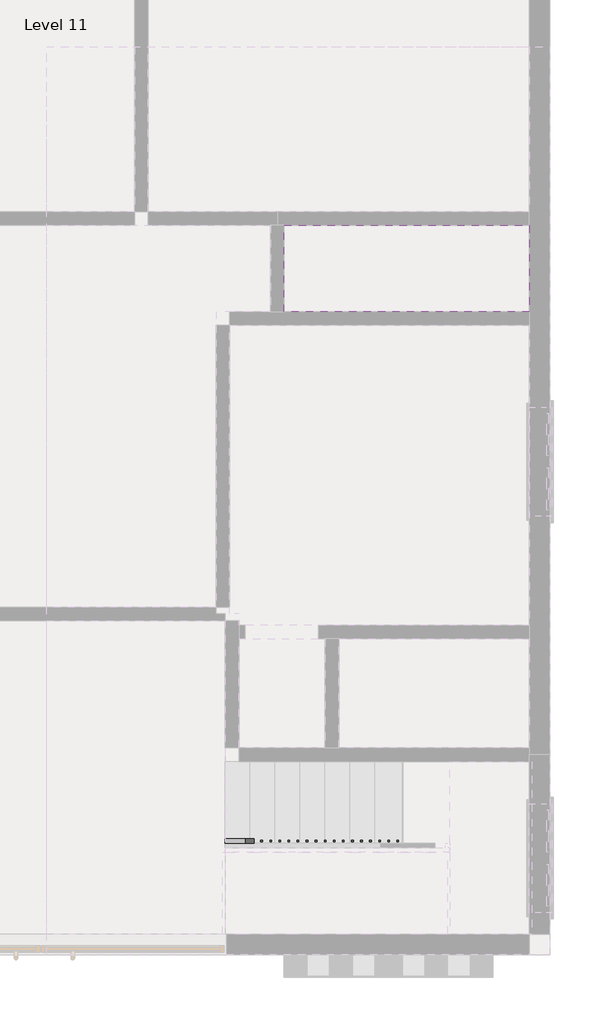
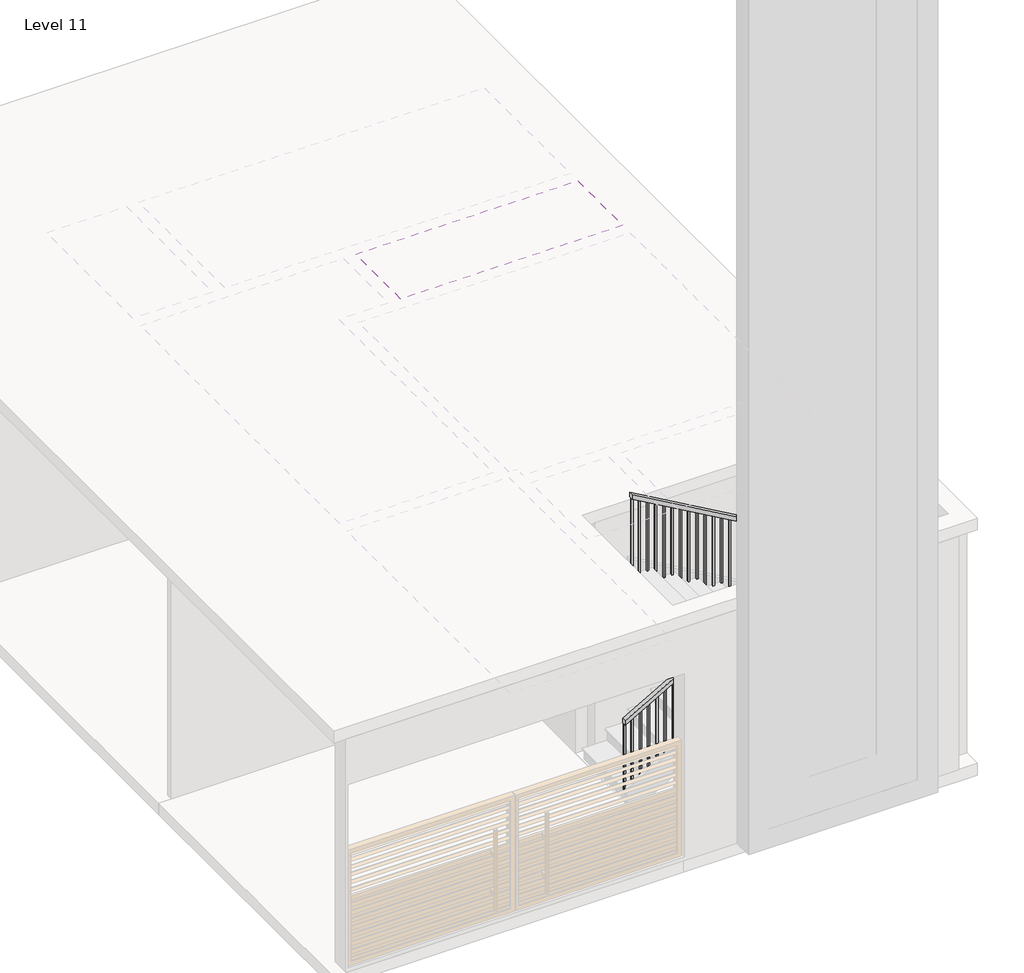
# One storey, part 2 of 3: 2 railings, 1 covering.
"""IFC4 building model written with IfcOpenShell, lengths in millimetres."""

from ifc_helpers import new_model, si_unit, frame, origin, place, context, project, spatial, polyline, outline, extrude, faceted_brep, element, save

model = new_model("IFC4")

# Units and contexts
model_context = context("Model", 3, world=origin())
ifc_project = project(units=[si_unit("LENGTHUNIT", "METRE", prefix="MILLI")], contexts=[model_context])

# Site, building, storey
site = spatial("IfcSite", under=ifc_project)
building = spatial("IfcBuilding", under=site)
storey = spatial("IfcBuildingStorey", under=building, Name="Level 11", Elevation=0.0)

# Covering
placement = place(None, origin())
element("IfcCovering", 1, ObjectType="2' x 4' ACT System", at=placement, inside=storey, context=model_context, shape_type="SweptSolid", body=[
    extrude(outline(polyline([(-930.7154463, 2171.4455275), (1812.4845537, 2171.4455275), (1812.4845537, 1206.2455275), (-930.7154463, 1206.2455275), (-930.7154463, 2171.4455275)])), frame((0.0, 0.0, 2743.2), z_axis=(0.0, 0.0, 1.0), x_axis=(1.0, 0.0, 0.0)), (0.0, 0.0, 1.0), 57.15),
])

# Railings
element("IfcRailing", 2, ObjectType="Handrail - Rectangular", at=placement, inside=storey, context=model_context, shape_type="SolidModel", body=[
    faceted_brep([(-1591.1154463, -4686.5544725, 1074.42), (-1591.1154463, -4686.5544725, 1015.8782835), (-1591.1154463, -4737.3544725, 1015.8782835), (-1591.1154463, -4737.3544725, 1074.42), (847.2845537, -4686.5544725, 2470.9581818), (898.0845537, -4686.5544725, 2441.5110107), (898.0845537, -4737.3544725, 2441.5110107), (847.2845537, -4737.3544725, 2470.9581818), (847.2845537, -4686.5544725, 2514.6), (898.0845537, -4686.5544725, 2463.8), (898.0845537, -4737.3544725, 2463.8), (847.2845537, -4737.3544725, 2514.6), (974.2845537, -4686.5544725, 2514.6), (974.2845537, -4686.5544725, 2463.8), (923.4845537, -4737.3544725, 2463.8), (923.4845537, -4737.3544725, 2514.6), (974.2845537, -4813.5544725, 2514.6), (974.2845537, -4813.5544725, 2463.8), (923.4845537, -4813.5544725, 2463.8), (923.4845537, -4813.5544725, 2514.6), (974.2845537, -4838.9544725, 2514.6), (923.4845537, -4838.9544725, 2514.6), (923.4845537, -4889.7544725, 2463.8), (974.2845537, -4889.7544725, 2463.8)], [[[0, 1, 2, 3]], [[1, 0, 4, 5]], [[2, 1, 5, 6]], [[3, 2, 6, 7]], [[0, 3, 7, 4]], [[5, 4, 8, 9]], [[6, 5, 9, 10]], [[7, 6, 10, 11]], [[4, 7, 11, 8]], [[9, 8, 12, 13]], [[10, 9, 13, 14]], [[11, 10, 14, 15]], [[8, 11, 15, 12]], [[13, 12, 16, 17]], [[14, 13, 17, 18]], [[15, 14, 18, 19]], [[12, 15, 19, 16]], [[20, 21, 22, 23]], [[17, 16, 20, 23]], [[18, 17, 23, 22]], [[19, 18, 22, 21]], [[16, 19, 21, 20]]]),
    faceted_brep([(974.2845537, -4838.9544725, 2514.6), (974.2845537, -4889.7544725, 2463.8), (923.4845537, -4889.7544725, 2463.8), (923.4845537, -4838.9544725, 2514.6), (974.2845537, -4838.9544725, 2645.5254545), (923.4845537, -4838.9544725, 2616.0782835), (923.4845537, -4889.7544725, 2616.0782835), (974.2845537, -4889.7544725, 2645.5254545)], [[[0, 1, 2, 3]], [[4, 5, 6, 7]], [[1, 0, 4, 7]], [[2, 1, 7, 6]], [[3, 2, 6, 5]], [[0, 3, 5, 4]]]),
    faceted_brep([(974.2845537, -4889.7544725, 2645.5254545), (923.4845537, -4889.7544725, 2616.0782835), (923.4845537, -4838.9544725, 2616.0782835), (974.2845537, -4838.9544725, 2645.5254545), (-1591.1154463, -4889.7544725, 4114.8), (-1591.1154463, -4838.9544725, 4114.8), (-1591.1154463, -4838.9544725, 4056.2582835), (-1591.1154463, -4889.7544725, 4056.2582835)], [[[0, 1, 2, 3]], [[4, 5, 6, 7]], [[1, 0, 4, 7]], [[2, 1, 7, 6]], [[3, 2, 6, 5]], [[0, 3, 5, 4]]]),
    extrude(outline(polyline([(3992.6139653, -1479.9904463), (4003.5244198, -1499.0404463), (3040.38, -1499.0404463), (3040.38, -1479.9904463), (3992.6139653, -1479.9904463)])), frame((0.0, -4873.8794725, 0.0), z_axis=(0.0, 1.0, 0.0), x_axis=(0.0, 0.0, 1.0)), (0.0, 0.0, 1.0), 19.05),
    extrude(outline(polyline([(3934.4248744, -1378.3904463), (3945.3353289, -1397.4404463), (3040.38, -1397.4404463), (3040.38, -1378.3904463), (3934.4248744, -1378.3904463)])), frame((0.0, -4873.8794725, 0.0), z_axis=(0.0, 1.0, 0.0), x_axis=(0.0, 0.0, 1.0)), (0.0, 0.0, 1.0), 19.05),
    extrude(outline(polyline([(3876.2357835, -1276.7904463), (3887.146238, -1295.8404463), (2880.36, -1295.8404463), (2880.36, -1276.7904463), (3876.2357835, -1276.7904463)])), frame((0.0, -4873.8794725, 0.0), z_axis=(0.0, 1.0, 0.0), x_axis=(0.0, 0.0, 1.0)), (0.0, 0.0, 1.0), 19.05),
    extrude(outline(polyline([(3818.0466926, -1175.1904463), (3828.9571471, -1194.2404463), (2880.36, -1194.2404463), (2880.36, -1175.1904463), (3818.0466926, -1175.1904463)])), frame((0.0, -4873.8794725, 0.0), z_axis=(0.0, 1.0, 0.0), x_axis=(0.0, 0.0, 1.0)), (0.0, 0.0, 1.0), 19.05),
    extrude(outline(polyline([(3759.8576016, -1073.5904463), (3770.7680562, -1092.6404463), (2880.36, -1092.6404463), (2880.36, -1073.5904463), (3759.8576016, -1073.5904463)])), frame((0.0, -4873.8794725, 0.0), z_axis=(0.0, 1.0, 0.0), x_axis=(0.0, 0.0, 1.0)), (0.0, 0.0, 1.0), 19.05),
    extrude(outline(polyline([(3701.6685107, -971.9904463), (3712.5789653, -991.0404463), (2720.34, -991.0404463), (2720.34, -971.9904463), (3701.6685107, -971.9904463)])), frame((0.0, -4873.8794725, 0.0), z_axis=(0.0, 1.0, 0.0), x_axis=(0.0, 0.0, 1.0)), (0.0, 0.0, 1.0), 19.05),
    extrude(outline(polyline([(3643.4794198, -870.3904463), (3654.3898744, -889.4404463), (2720.34, -889.4404463), (2720.34, -870.3904463), (3643.4794198, -870.3904463)])), frame((0.0, -4873.8794725, 0.0), z_axis=(0.0, 1.0, 0.0), x_axis=(0.0, 0.0, 1.0)), (0.0, 0.0, 1.0), 19.05),
    extrude(outline(polyline([(3585.2903289, -768.7904463), (3596.2007835, -787.8404463), (2720.34, -787.8404463), (2720.34, -768.7904463), (3585.2903289, -768.7904463)])), frame((0.0, -4873.8794725, 0.0), z_axis=(0.0, 1.0, 0.0), x_axis=(0.0, 0.0, 1.0)), (0.0, 0.0, 1.0), 19.05),
    extrude(outline(polyline([(3527.101238, -667.1904463), (3538.0116926, -686.2404463), (2560.32, -686.2404463), (2560.32, -667.1904463), (3527.101238, -667.1904463)])), frame((0.0, -4873.8794725, 0.0), z_axis=(0.0, 1.0, 0.0), x_axis=(0.0, 0.0, 1.0)), (0.0, 0.0, 1.0), 19.05),
    extrude(outline(polyline([(3468.9121471, -565.5904463), (3479.8226016, -584.6404463), (2560.32, -584.6404463), (2560.32, -565.5904463), (3468.9121471, -565.5904463)])), frame((0.0, -4873.8794725, 0.0), z_axis=(0.0, 1.0, 0.0), x_axis=(0.0, 0.0, 1.0)), (0.0, 0.0, 1.0), 19.05),
    extrude(outline(polyline([(3410.7230562, -463.9904463), (3421.6335107, -483.0404463), (2560.32, -483.0404463), (2560.32, -463.9904463), (3410.7230562, -463.9904463)])), frame((0.0, -4873.8794725, 0.0), z_axis=(0.0, 1.0, 0.0), x_axis=(0.0, 0.0, 1.0)), (0.0, 0.0, 1.0), 19.05),
    extrude(outline(polyline([(3352.5339653, -362.3904463), (3363.4444198, -381.4404463), (2400.3, -381.4404463), (2400.3, -362.3904463), (3352.5339653, -362.3904463)])), frame((0.0, -4873.8794725, 0.0), z_axis=(0.0, 1.0, 0.0), x_axis=(0.0, 0.0, 1.0)), (0.0, 0.0, 1.0), 19.05),
    extrude(outline(polyline([(3294.3448744, -260.7904463), (3305.2553289, -279.8404463), (2400.3, -279.8404463), (2400.3, -260.7904463), (3294.3448744, -260.7904463)])), frame((0.0, -4873.8794725, 0.0), z_axis=(0.0, 1.0, 0.0), x_axis=(0.0, 0.0, 1.0)), (0.0, 0.0, 1.0), 19.05),
    extrude(outline(polyline([(3236.1557835, -159.1904463), (3247.066238, -178.2404463), (2240.28, -178.2404463), (2240.28, -159.1904463), (3236.1557835, -159.1904463)])), frame((0.0, -4873.8794725, 0.0), z_axis=(0.0, 1.0, 0.0), x_axis=(0.0, 0.0, 1.0)), (0.0, 0.0, 1.0), 19.05),
    extrude(outline(polyline([(3177.9666926, -57.5904463), (3188.8771471, -76.6404463), (2240.28, -76.6404463), (2240.28, -57.5904463), (3177.9666926, -57.5904463)])), frame((0.0, -4873.8794725, 0.0), z_axis=(0.0, 1.0, 0.0), x_axis=(0.0, 0.0, 1.0)), (0.0, 0.0, 1.0), 19.05),
    extrude(outline(polyline([(3119.7776016, 44.0095537), (3130.6880562, 24.9595537), (2240.28, 24.9595537), (2240.28, 44.0095537), (3119.7776016, 44.0095537)])), frame((0.0, -4873.8794725, 0.0), z_axis=(0.0, 1.0, 0.0), x_axis=(0.0, 0.0, 1.0)), (0.0, 0.0, 1.0), 19.05),
    extrude(outline(polyline([(3061.5885107, 145.6095537), (3072.4989653, 126.5595537), (2080.26, 126.5595537), (2080.26, 145.6095537), (3061.5885107, 145.6095537)])), frame((0.0, -4873.8794725, 0.0), z_axis=(0.0, 1.0, 0.0), x_axis=(0.0, 0.0, 1.0)), (0.0, 0.0, 1.0), 19.05),
    extrude(outline(polyline([(3003.3994198, 247.2095537), (3014.3098744, 228.1595537), (2080.26, 228.1595537), (2080.26, 247.2095537), (3003.3994198, 247.2095537)])), frame((0.0, -4873.8794725, 0.0), z_axis=(0.0, 1.0, 0.0), x_axis=(0.0, 0.0, 1.0)), (0.0, 0.0, 1.0), 19.05),
    extrude(outline(polyline([(2945.2103289, 348.8095537), (2956.1207835, 329.7595537), (2080.26, 329.7595537), (2080.26, 348.8095537), (2945.2103289, 348.8095537)])), frame((0.0, -4873.8794725, 0.0), z_axis=(0.0, 1.0, 0.0), x_axis=(0.0, 0.0, 1.0)), (0.0, 0.0, 1.0), 19.05),
    extrude(outline(polyline([(2887.021238, 450.4095537), (2897.9316926, 431.3595537), (1920.24, 431.3595537), (1920.24, 450.4095537), (2887.021238, 450.4095537)])), frame((0.0, -4873.8794725, 0.0), z_axis=(0.0, 1.0, 0.0), x_axis=(0.0, 0.0, 1.0)), (0.0, 0.0, 1.0), 19.05),
    extrude(outline(polyline([(2828.8321471, 552.0095537), (2839.7426016, 532.9595537), (1920.24, 532.9595537), (1920.24, 552.0095537), (2828.8321471, 552.0095537)])), frame((0.0, -4873.8794725, 0.0), z_axis=(0.0, 1.0, 0.0), x_axis=(0.0, 0.0, 1.0)), (0.0, 0.0, 1.0), 19.05),
    extrude(outline(polyline([(2770.6430562, 653.6095537), (2781.5535107, 634.5595537), (1920.24, 634.5595537), (1920.24, 653.6095537), (2770.6430562, 653.6095537)])), frame((0.0, -4873.8794725, 0.0), z_axis=(0.0, 1.0, 0.0), x_axis=(0.0, 0.0, 1.0)), (0.0, 0.0, 1.0), 19.05),
    extrude(outline(polyline([(2712.4539653, 755.2095537), (2723.3644198, 736.1595537), (1760.22, 736.1595537), (1760.22, 755.2095537), (2712.4539653, 755.2095537)])), frame((0.0, -4873.8794725, 0.0), z_axis=(0.0, 1.0, 0.0), x_axis=(0.0, 0.0, 1.0)), (0.0, 0.0, 1.0), 19.05),
    extrude(outline(polyline([(2654.2648744, 856.8095537), (2665.1753289, 837.7595537), (1760.22, 837.7595537), (1760.22, 856.8095537), (2654.2648744, 856.8095537)])), frame((0.0, -4873.8794725, 0.0), z_axis=(0.0, 1.0, 0.0), x_axis=(0.0, 0.0, 1.0)), (0.0, 0.0, 1.0), 19.05),
    extrude(outline(polyline([(939.3595537, -4804.0294725), (958.4095537, -4804.0294725), (958.4095537, -4823.0794725), (939.3595537, -4823.0794725), (939.3595537, -4804.0294725)])), frame((0.0, 0.0, 1600.2), z_axis=(0.0, 0.0, 1.0), x_axis=(1.0, 0.0, 0.0)), (0.0, 0.0, 1.0), 863.6),
    extrude(outline(polyline([(2417.8716926, 856.8095537), (2406.961238, 837.7595537), (1440.18, 837.7595537), (1440.18, 856.8095537), (2417.8716926, 856.8095537)])), frame((0.0, -4721.4794725, 0.0), z_axis=(0.0, 1.0, 0.0), x_axis=(0.0, 0.0, 1.0)), (0.0, 0.0, 1.0), 19.05),
    extrude(outline(polyline([(2359.6826016, 755.2095537), (2348.7721471, 736.1595537), (1440.18, 736.1595537), (1440.18, 755.2095537), (2359.6826016, 755.2095537)])), frame((0.0, -4721.4794725, 0.0), z_axis=(0.0, 1.0, 0.0), x_axis=(0.0, 0.0, 1.0)), (0.0, 0.0, 1.0), 19.05),
    extrude(outline(polyline([(2301.4935107, 653.6095537), (2290.5830562, 634.5595537), (1440.18, 634.5595537), (1440.18, 653.6095537), (2301.4935107, 653.6095537)])), frame((0.0, -4721.4794725, 0.0), z_axis=(0.0, 1.0, 0.0), x_axis=(0.0, 0.0, 1.0)), (0.0, 0.0, 1.0), 19.05),
    extrude(outline(polyline([(2243.3044198, 552.0095537), (2232.3939653, 532.9595537), (1280.16, 532.9595537), (1280.16, 552.0095537), (2243.3044198, 552.0095537)])), frame((0.0, -4721.4794725, 0.0), z_axis=(0.0, 1.0, 0.0), x_axis=(0.0, 0.0, 1.0)), (0.0, 0.0, 1.0), 19.05),
    extrude(outline(polyline([(2185.1153289, 450.4095537), (2174.2048744, 431.3595537), (1280.16, 431.3595537), (1280.16, 450.4095537), (2185.1153289, 450.4095537)])), frame((0.0, -4721.4794725, 0.0), z_axis=(0.0, 1.0, 0.0), x_axis=(0.0, 0.0, 1.0)), (0.0, 0.0, 1.0), 19.05),
    extrude(outline(polyline([(2126.926238, 348.8095537), (2116.0157835, 329.7595537), (1120.14, 329.7595537), (1120.14, 348.8095537), (2126.926238, 348.8095537)])), frame((0.0, -4721.4794725, 0.0), z_axis=(0.0, 1.0, 0.0), x_axis=(0.0, 0.0, 1.0)), (0.0, 0.0, 1.0), 19.05),
    extrude(outline(polyline([(2068.7371471, 247.2095537), (2057.8266926, 228.1595537), (1120.14, 228.1595537), (1120.14, 247.2095537), (2068.7371471, 247.2095537)])), frame((0.0, -4721.4794725, 0.0), z_axis=(0.0, 1.0, 0.0), x_axis=(0.0, 0.0, 1.0)), (0.0, 0.0, 1.0), 19.05),
    extrude(outline(polyline([(2010.5480562, 145.6095537), (1999.6376016, 126.5595537), (1120.14, 126.5595537), (1120.14, 145.6095537), (2010.5480562, 145.6095537)])), frame((0.0, -4721.4794725, 0.0), z_axis=(0.0, 1.0, 0.0), x_axis=(0.0, 0.0, 1.0)), (0.0, 0.0, 1.0), 19.05),
    extrude(outline(polyline([(1952.3589653, 44.0095537), (1941.4485107, 24.9595537), (960.12, 24.9595537), (960.12, 44.0095537), (1952.3589653, 44.0095537)])), frame((0.0, -4721.4794725, 0.0), z_axis=(0.0, 1.0, 0.0), x_axis=(0.0, 0.0, 1.0)), (0.0, 0.0, 1.0), 19.05),
    extrude(outline(polyline([(1894.1698744, -57.5904463), (1883.2594198, -76.6404463), (960.12, -76.6404463), (960.12, -57.5904463), (1894.1698744, -57.5904463)])), frame((0.0, -4721.4794725, 0.0), z_axis=(0.0, 1.0, 0.0), x_axis=(0.0, 0.0, 1.0)), (0.0, 0.0, 1.0), 19.05),
    extrude(outline(polyline([(1835.9807835, -159.1904463), (1825.0703289, -178.2404463), (960.12, -178.2404463), (960.12, -159.1904463), (1835.9807835, -159.1904463)])), frame((0.0, -4721.4794725, 0.0), z_axis=(0.0, 1.0, 0.0), x_axis=(0.0, 0.0, 1.0)), (0.0, 0.0, 1.0), 19.05),
    extrude(outline(polyline([(1777.7916926, -260.7904463), (1766.881238, -279.8404463), (800.1, -279.8404463), (800.1, -260.7904463), (1777.7916926, -260.7904463)])), frame((0.0, -4721.4794725, 0.0), z_axis=(0.0, 1.0, 0.0), x_axis=(0.0, 0.0, 1.0)), (0.0, 0.0, 1.0), 19.05),
    extrude(outline(polyline([(1719.6026016, -362.3904463), (1708.6921471, -381.4404463), (800.1, -381.4404463), (800.1, -362.3904463), (1719.6026016, -362.3904463)])), frame((0.0, -4721.4794725, 0.0), z_axis=(0.0, 1.0, 0.0), x_axis=(0.0, 0.0, 1.0)), (0.0, 0.0, 1.0), 19.05),
    extrude(outline(polyline([(1661.4135107, -463.9904463), (1650.5030562, -483.0404463), (800.1, -483.0404463), (800.1, -463.9904463), (1661.4135107, -463.9904463)])), frame((0.0, -4721.4794725, 0.0), z_axis=(0.0, 1.0, 0.0), x_axis=(0.0, 0.0, 1.0)), (0.0, 0.0, 1.0), 19.05),
    extrude(outline(polyline([(1603.2244198, -565.5904463), (1592.3139653, -584.6404463), (640.08, -584.6404463), (640.08, -565.5904463), (1603.2244198, -565.5904463)])), frame((0.0, -4721.4794725, 0.0), z_axis=(0.0, 1.0, 0.0), x_axis=(0.0, 0.0, 1.0)), (0.0, 0.0, 1.0), 19.05),
    extrude(outline(polyline([(1545.0353289, -667.1904463), (1534.1248744, -686.2404463), (640.08, -686.2404463), (640.08, -667.1904463), (1545.0353289, -667.1904463)])), frame((0.0, -4721.4794725, 0.0), z_axis=(0.0, 1.0, 0.0), x_axis=(0.0, 0.0, 1.0)), (0.0, 0.0, 1.0), 19.05),
    extrude(outline(polyline([(1486.846238, -768.7904463), (1475.9357835, -787.8404463), (480.06, -787.8404463), (480.06, -768.7904463), (1486.846238, -768.7904463)])), frame((0.0, -4721.4794725, 0.0), z_axis=(0.0, 1.0, 0.0), x_axis=(0.0, 0.0, 1.0)), (0.0, 0.0, 1.0), 19.05),
    extrude(outline(polyline([(1428.6571471, -870.3904463), (1417.7466926, -889.4404463), (480.06, -889.4404463), (480.06, -870.3904463), (1428.6571471, -870.3904463)])), frame((0.0, -4721.4794725, 0.0), z_axis=(0.0, 1.0, 0.0), x_axis=(0.0, 0.0, 1.0)), (0.0, 0.0, 1.0), 19.05),
    extrude(outline(polyline([(1370.4680562, -971.9904463), (1359.5576016, -991.0404463), (480.06, -991.0404463), (480.06, -971.9904463), (1370.4680562, -971.9904463)])), frame((0.0, -4721.4794725, 0.0), z_axis=(0.0, 1.0, 0.0), x_axis=(0.0, 0.0, 1.0)), (0.0, 0.0, 1.0), 19.05),
    extrude(outline(polyline([(1312.2789653, -1073.5904463), (1301.3685107, -1092.6404463), (320.04, -1092.6404463), (320.04, -1073.5904463), (1312.2789653, -1073.5904463)])), frame((0.0, -4721.4794725, 0.0), z_axis=(0.0, 1.0, 0.0), x_axis=(0.0, 0.0, 1.0)), (0.0, 0.0, 1.0), 19.05),
    extrude(outline(polyline([(1254.0898744, -1175.1904463), (1243.1794198, -1194.2404463), (320.04, -1194.2404463), (320.04, -1175.1904463), (1254.0898744, -1175.1904463)])), frame((0.0, -4721.4794725, 0.0), z_axis=(0.0, 1.0, 0.0), x_axis=(0.0, 0.0, 1.0)), (0.0, 0.0, 1.0), 19.05),
    extrude(outline(polyline([(1195.9007835, -1276.7904463), (1184.9903289, -1295.8404463), (320.04, -1295.8404463), (320.04, -1276.7904463), (1195.9007835, -1276.7904463)])), frame((0.0, -4721.4794725, 0.0), z_axis=(0.0, 1.0, 0.0), x_axis=(0.0, 0.0, 1.0)), (0.0, 0.0, 1.0), 19.05),
    extrude(outline(polyline([(1137.7116926, -1378.3904463), (1126.801238, -1397.4404463), (160.02, -1397.4404463), (160.02, -1378.3904463), (1137.7116926, -1378.3904463)])), frame((0.0, -4721.4794725, 0.0), z_axis=(0.0, 1.0, 0.0), x_axis=(0.0, 0.0, 1.0)), (0.0, 0.0, 1.0), 19.05),
    extrude(outline(polyline([(1079.5226016, -1479.9904463), (1068.6121471, -1499.0404463), (160.02, -1499.0404463), (160.02, -1479.9904463), (1079.5226016, -1479.9904463)])), frame((0.0, -4721.4794725, 0.0), z_axis=(0.0, 1.0, 0.0), x_axis=(0.0, 0.0, 1.0)), (0.0, 0.0, 1.0), 19.05),
    extrude(outline(polyline([(939.3595537, -4854.8294725), (958.4095537, -4854.8294725), (958.4095537, -4873.8794725), (939.3595537, -4873.8794725), (939.3595537, -4854.8294725)])), frame((0.0, 0.0, 1600.2), z_axis=(0.0, 0.0, 1.0), x_axis=(1.0, 0.0, 0.0)), (0.0, 0.0, 1.0), 863.6),
    extrude(outline(polyline([(939.3595537, -4721.4794725), (939.3595537, -4702.4294725), (958.4095537, -4702.4294725), (958.4095537, -4721.4794725), (939.3595537, -4721.4794725)])), frame((0.0, 0.0, 1600.2), z_axis=(0.0, 0.0, 1.0), x_axis=(1.0, 0.0, 0.0)), (0.0, 0.0, 1.0), 863.6),
    extrude(outline(polyline([(4045.3478289, -1572.0654463), (4056.2582835, -1591.1154463), (3040.38, -1591.1154463), (3040.38, -1572.0654463), (4045.3478289, -1572.0654463)])), frame((0.0, -4873.8794725, 0.0), z_axis=(0.0, 1.0, 0.0), x_axis=(0.0, 0.0, 1.0)), (0.0, 0.0, 1.0), 19.05),
    extrude(outline(polyline([(1026.788738, -1572.0654463), (1015.8782835, -1591.1154463), (160.02, -1591.1154463), (160.02, -1572.0654463), (1026.788738, -1572.0654463)])), frame((0.0, -4721.4794725, 0.0), z_axis=(0.0, 1.0, 0.0), x_axis=(0.0, 0.0, 1.0)), (0.0, 0.0, 1.0), 19.05),
])
element("IfcRailing", 3, ObjectType="Handrail - Rectangular", at=placement, inside=storey, context=model_context, shape_type="SolidModel", body=[
    faceted_brep([(-1591.1154463, -4686.5544725, 1074.42), (-1591.1154463, -4686.5544725, 1015.8782835), (-1591.1154463, -4737.3544725, 1015.8782835), (-1591.1154463, -4737.3544725, 1074.42), (847.2845537, -4686.5544725, 2470.9581818), (898.0845537, -4686.5544725, 2441.5110107), (898.0845537, -4737.3544725, 2441.5110107), (847.2845537, -4737.3544725, 2470.9581818), (847.2845537, -4686.5544725, 2514.6), (898.0845537, -4686.5544725, 2463.8), (898.0845537, -4737.3544725, 2463.8), (847.2845537, -4737.3544725, 2514.6), (974.2845537, -4686.5544725, 2514.6), (974.2845537, -4686.5544725, 2463.8), (923.4845537, -4737.3544725, 2463.8), (923.4845537, -4737.3544725, 2514.6), (974.2845537, -4813.5544725, 2514.6), (974.2845537, -4813.5544725, 2463.8), (923.4845537, -4813.5544725, 2463.8), (923.4845537, -4813.5544725, 2514.6), (974.2845537, -4838.9544725, 2514.6), (923.4845537, -4838.9544725, 2514.6), (923.4845537, -4889.7544725, 2463.8), (974.2845537, -4889.7544725, 2463.8)], [[[0, 1, 2, 3]], [[1, 0, 4, 5]], [[2, 1, 5, 6]], [[3, 2, 6, 7]], [[0, 3, 7, 4]], [[5, 4, 8, 9]], [[6, 5, 9, 10]], [[7, 6, 10, 11]], [[4, 7, 11, 8]], [[9, 8, 12, 13]], [[10, 9, 13, 14]], [[11, 10, 14, 15]], [[8, 11, 15, 12]], [[13, 12, 16, 17]], [[14, 13, 17, 18]], [[15, 14, 18, 19]], [[12, 15, 19, 16]], [[20, 21, 22, 23]], [[17, 16, 20, 23]], [[18, 17, 23, 22]], [[19, 18, 22, 21]], [[16, 19, 21, 20]]]),
    faceted_brep([(974.2845537, -4838.9544725, 2514.6), (974.2845537, -4889.7544725, 2463.8), (923.4845537, -4889.7544725, 2463.8), (923.4845537, -4838.9544725, 2514.6), (974.2845537, -4838.9544725, 2645.5254545), (923.4845537, -4838.9544725, 2616.0782835), (923.4845537, -4889.7544725, 2616.0782835), (974.2845537, -4889.7544725, 2645.5254545)], [[[0, 1, 2, 3]], [[4, 5, 6, 7]], [[1, 0, 4, 7]], [[2, 1, 7, 6]], [[3, 2, 6, 5]], [[0, 3, 5, 4]]]),
    faceted_brep([(974.2845537, -4889.7544725, 2645.5254545), (923.4845537, -4889.7544725, 2616.0782835), (923.4845537, -4838.9544725, 2616.0782835), (974.2845537, -4838.9544725, 2645.5254545), (-1591.1154463, -4889.7544725, 4114.8), (-1591.1154463, -4838.9544725, 4114.8), (-1591.1154463, -4838.9544725, 4056.2582835), (-1591.1154463, -4889.7544725, 4056.2582835)], [[[0, 1, 2, 3]], [[4, 5, 6, 7]], [[1, 0, 4, 7]], [[2, 1, 7, 6]], [[3, 2, 6, 5]], [[0, 3, 5, 4]]]),
    extrude(outline(polyline([(3992.6139653, -1479.9904463), (4003.5244198, -1499.0404463), (3040.38, -1499.0404463), (3040.38, -1479.9904463), (3992.6139653, -1479.9904463)])), frame((0.0, -4873.8794725, 0.0), z_axis=(0.0, 1.0, 0.0), x_axis=(0.0, 0.0, 1.0)), (0.0, 0.0, 1.0), 19.05),
    extrude(outline(polyline([(3934.4248744, -1378.3904463), (3945.3353289, -1397.4404463), (3040.38, -1397.4404463), (3040.38, -1378.3904463), (3934.4248744, -1378.3904463)])), frame((0.0, -4873.8794725, 0.0), z_axis=(0.0, 1.0, 0.0), x_axis=(0.0, 0.0, 1.0)), (0.0, 0.0, 1.0), 19.05),
    extrude(outline(polyline([(3876.2357835, -1276.7904463), (3887.146238, -1295.8404463), (2880.36, -1295.8404463), (2880.36, -1276.7904463), (3876.2357835, -1276.7904463)])), frame((0.0, -4873.8794725, 0.0), z_axis=(0.0, 1.0, 0.0), x_axis=(0.0, 0.0, 1.0)), (0.0, 0.0, 1.0), 19.05),
    extrude(outline(polyline([(3818.0466926, -1175.1904463), (3828.9571471, -1194.2404463), (2880.36, -1194.2404463), (2880.36, -1175.1904463), (3818.0466926, -1175.1904463)])), frame((0.0, -4873.8794725, 0.0), z_axis=(0.0, 1.0, 0.0), x_axis=(0.0, 0.0, 1.0)), (0.0, 0.0, 1.0), 19.05),
    extrude(outline(polyline([(3759.8576016, -1073.5904463), (3770.7680562, -1092.6404463), (2880.36, -1092.6404463), (2880.36, -1073.5904463), (3759.8576016, -1073.5904463)])), frame((0.0, -4873.8794725, 0.0), z_axis=(0.0, 1.0, 0.0), x_axis=(0.0, 0.0, 1.0)), (0.0, 0.0, 1.0), 19.05),
    extrude(outline(polyline([(3701.6685107, -971.9904463), (3712.5789653, -991.0404463), (2720.34, -991.0404463), (2720.34, -971.9904463), (3701.6685107, -971.9904463)])), frame((0.0, -4873.8794725, 0.0), z_axis=(0.0, 1.0, 0.0), x_axis=(0.0, 0.0, 1.0)), (0.0, 0.0, 1.0), 19.05),
    extrude(outline(polyline([(3643.4794198, -870.3904463), (3654.3898744, -889.4404463), (2720.34, -889.4404463), (2720.34, -870.3904463), (3643.4794198, -870.3904463)])), frame((0.0, -4873.8794725, 0.0), z_axis=(0.0, 1.0, 0.0), x_axis=(0.0, 0.0, 1.0)), (0.0, 0.0, 1.0), 19.05),
    extrude(outline(polyline([(3585.2903289, -768.7904463), (3596.2007835, -787.8404463), (2720.34, -787.8404463), (2720.34, -768.7904463), (3585.2903289, -768.7904463)])), frame((0.0, -4873.8794725, 0.0), z_axis=(0.0, 1.0, 0.0), x_axis=(0.0, 0.0, 1.0)), (0.0, 0.0, 1.0), 19.05),
    extrude(outline(polyline([(3527.101238, -667.1904463), (3538.0116926, -686.2404463), (2560.32, -686.2404463), (2560.32, -667.1904463), (3527.101238, -667.1904463)])), frame((0.0, -4873.8794725, 0.0), z_axis=(0.0, 1.0, 0.0), x_axis=(0.0, 0.0, 1.0)), (0.0, 0.0, 1.0), 19.05),
    extrude(outline(polyline([(3468.9121471, -565.5904463), (3479.8226016, -584.6404463), (2560.32, -584.6404463), (2560.32, -565.5904463), (3468.9121471, -565.5904463)])), frame((0.0, -4873.8794725, 0.0), z_axis=(0.0, 1.0, 0.0), x_axis=(0.0, 0.0, 1.0)), (0.0, 0.0, 1.0), 19.05),
    extrude(outline(polyline([(3410.7230562, -463.9904463), (3421.6335107, -483.0404463), (2560.32, -483.0404463), (2560.32, -463.9904463), (3410.7230562, -463.9904463)])), frame((0.0, -4873.8794725, 0.0), z_axis=(0.0, 1.0, 0.0), x_axis=(0.0, 0.0, 1.0)), (0.0, 0.0, 1.0), 19.05),
    extrude(outline(polyline([(3352.5339653, -362.3904463), (3363.4444198, -381.4404463), (2400.3, -381.4404463), (2400.3, -362.3904463), (3352.5339653, -362.3904463)])), frame((0.0, -4873.8794725, 0.0), z_axis=(0.0, 1.0, 0.0), x_axis=(0.0, 0.0, 1.0)), (0.0, 0.0, 1.0), 19.05),
    extrude(outline(polyline([(3294.3448744, -260.7904463), (3305.2553289, -279.8404463), (2400.3, -279.8404463), (2400.3, -260.7904463), (3294.3448744, -260.7904463)])), frame((0.0, -4873.8794725, 0.0), z_axis=(0.0, 1.0, 0.0), x_axis=(0.0, 0.0, 1.0)), (0.0, 0.0, 1.0), 19.05),
    extrude(outline(polyline([(3236.1557835, -159.1904463), (3247.066238, -178.2404463), (2240.28, -178.2404463), (2240.28, -159.1904463), (3236.1557835, -159.1904463)])), frame((0.0, -4873.8794725, 0.0), z_axis=(0.0, 1.0, 0.0), x_axis=(0.0, 0.0, 1.0)), (0.0, 0.0, 1.0), 19.05),
    extrude(outline(polyline([(3177.9666926, -57.5904463), (3188.8771471, -76.6404463), (2240.28, -76.6404463), (2240.28, -57.5904463), (3177.9666926, -57.5904463)])), frame((0.0, -4873.8794725, 0.0), z_axis=(0.0, 1.0, 0.0), x_axis=(0.0, 0.0, 1.0)), (0.0, 0.0, 1.0), 19.05),
    extrude(outline(polyline([(3119.7776016, 44.0095537), (3130.6880562, 24.9595537), (2240.28, 24.9595537), (2240.28, 44.0095537), (3119.7776016, 44.0095537)])), frame((0.0, -4873.8794725, 0.0), z_axis=(0.0, 1.0, 0.0), x_axis=(0.0, 0.0, 1.0)), (0.0, 0.0, 1.0), 19.05),
    extrude(outline(polyline([(3061.5885107, 145.6095537), (3072.4989653, 126.5595537), (2080.26, 126.5595537), (2080.26, 145.6095537), (3061.5885107, 145.6095537)])), frame((0.0, -4873.8794725, 0.0), z_axis=(0.0, 1.0, 0.0), x_axis=(0.0, 0.0, 1.0)), (0.0, 0.0, 1.0), 19.05),
    extrude(outline(polyline([(3003.3994198, 247.2095537), (3014.3098744, 228.1595537), (2080.26, 228.1595537), (2080.26, 247.2095537), (3003.3994198, 247.2095537)])), frame((0.0, -4873.8794725, 0.0), z_axis=(0.0, 1.0, 0.0), x_axis=(0.0, 0.0, 1.0)), (0.0, 0.0, 1.0), 19.05),
    extrude(outline(polyline([(2945.2103289, 348.8095537), (2956.1207835, 329.7595537), (2080.26, 329.7595537), (2080.26, 348.8095537), (2945.2103289, 348.8095537)])), frame((0.0, -4873.8794725, 0.0), z_axis=(0.0, 1.0, 0.0), x_axis=(0.0, 0.0, 1.0)), (0.0, 0.0, 1.0), 19.05),
    extrude(outline(polyline([(2887.021238, 450.4095537), (2897.9316926, 431.3595537), (1920.24, 431.3595537), (1920.24, 450.4095537), (2887.021238, 450.4095537)])), frame((0.0, -4873.8794725, 0.0), z_axis=(0.0, 1.0, 0.0), x_axis=(0.0, 0.0, 1.0)), (0.0, 0.0, 1.0), 19.05),
    extrude(outline(polyline([(2828.8321471, 552.0095537), (2839.7426016, 532.9595537), (1920.24, 532.9595537), (1920.24, 552.0095537), (2828.8321471, 552.0095537)])), frame((0.0, -4873.8794725, 0.0), z_axis=(0.0, 1.0, 0.0), x_axis=(0.0, 0.0, 1.0)), (0.0, 0.0, 1.0), 19.05),
    extrude(outline(polyline([(2770.6430562, 653.6095537), (2781.5535107, 634.5595537), (1920.24, 634.5595537), (1920.24, 653.6095537), (2770.6430562, 653.6095537)])), frame((0.0, -4873.8794725, 0.0), z_axis=(0.0, 1.0, 0.0), x_axis=(0.0, 0.0, 1.0)), (0.0, 0.0, 1.0), 19.05),
    extrude(outline(polyline([(2712.4539653, 755.2095537), (2723.3644198, 736.1595537), (1760.22, 736.1595537), (1760.22, 755.2095537), (2712.4539653, 755.2095537)])), frame((0.0, -4873.8794725, 0.0), z_axis=(0.0, 1.0, 0.0), x_axis=(0.0, 0.0, 1.0)), (0.0, 0.0, 1.0), 19.05),
    extrude(outline(polyline([(2654.2648744, 856.8095537), (2665.1753289, 837.7595537), (1760.22, 837.7595537), (1760.22, 856.8095537), (2654.2648744, 856.8095537)])), frame((0.0, -4873.8794725, 0.0), z_axis=(0.0, 1.0, 0.0), x_axis=(0.0, 0.0, 1.0)), (0.0, 0.0, 1.0), 19.05),
    extrude(outline(polyline([(939.3595537, -4804.0294725), (958.4095537, -4804.0294725), (958.4095537, -4823.0794725), (939.3595537, -4823.0794725), (939.3595537, -4804.0294725)])), frame((0.0, 0.0, 1600.2), z_axis=(0.0, 0.0, 1.0), x_axis=(1.0, 0.0, 0.0)), (0.0, 0.0, 1.0), 863.6),
    extrude(outline(polyline([(2417.8716926, 856.8095537), (2406.961238, 837.7595537), (1440.18, 837.7595537), (1440.18, 856.8095537), (2417.8716926, 856.8095537)])), frame((0.0, -4721.4794725, 0.0), z_axis=(0.0, 1.0, 0.0), x_axis=(0.0, 0.0, 1.0)), (0.0, 0.0, 1.0), 19.05),
    extrude(outline(polyline([(2359.6826016, 755.2095537), (2348.7721471, 736.1595537), (1440.18, 736.1595537), (1440.18, 755.2095537), (2359.6826016, 755.2095537)])), frame((0.0, -4721.4794725, 0.0), z_axis=(0.0, 1.0, 0.0), x_axis=(0.0, 0.0, 1.0)), (0.0, 0.0, 1.0), 19.05),
    extrude(outline(polyline([(2301.4935107, 653.6095537), (2290.5830562, 634.5595537), (1440.18, 634.5595537), (1440.18, 653.6095537), (2301.4935107, 653.6095537)])), frame((0.0, -4721.4794725, 0.0), z_axis=(0.0, 1.0, 0.0), x_axis=(0.0, 0.0, 1.0)), (0.0, 0.0, 1.0), 19.05),
    extrude(outline(polyline([(2243.3044198, 552.0095537), (2232.3939653, 532.9595537), (1280.16, 532.9595537), (1280.16, 552.0095537), (2243.3044198, 552.0095537)])), frame((0.0, -4721.4794725, 0.0), z_axis=(0.0, 1.0, 0.0), x_axis=(0.0, 0.0, 1.0)), (0.0, 0.0, 1.0), 19.05),
    extrude(outline(polyline([(2185.1153289, 450.4095537), (2174.2048744, 431.3595537), (1280.16, 431.3595537), (1280.16, 450.4095537), (2185.1153289, 450.4095537)])), frame((0.0, -4721.4794725, 0.0), z_axis=(0.0, 1.0, 0.0), x_axis=(0.0, 0.0, 1.0)), (0.0, 0.0, 1.0), 19.05),
    extrude(outline(polyline([(2126.926238, 348.8095537), (2116.0157835, 329.7595537), (1120.14, 329.7595537), (1120.14, 348.8095537), (2126.926238, 348.8095537)])), frame((0.0, -4721.4794725, 0.0), z_axis=(0.0, 1.0, 0.0), x_axis=(0.0, 0.0, 1.0)), (0.0, 0.0, 1.0), 19.05),
    extrude(outline(polyline([(2068.7371471, 247.2095537), (2057.8266926, 228.1595537), (1120.14, 228.1595537), (1120.14, 247.2095537), (2068.7371471, 247.2095537)])), frame((0.0, -4721.4794725, 0.0), z_axis=(0.0, 1.0, 0.0), x_axis=(0.0, 0.0, 1.0)), (0.0, 0.0, 1.0), 19.05),
    extrude(outline(polyline([(2010.5480562, 145.6095537), (1999.6376016, 126.5595537), (1120.14, 126.5595537), (1120.14, 145.6095537), (2010.5480562, 145.6095537)])), frame((0.0, -4721.4794725, 0.0), z_axis=(0.0, 1.0, 0.0), x_axis=(0.0, 0.0, 1.0)), (0.0, 0.0, 1.0), 19.05),
    extrude(outline(polyline([(1952.3589653, 44.0095537), (1941.4485107, 24.9595537), (960.12, 24.9595537), (960.12, 44.0095537), (1952.3589653, 44.0095537)])), frame((0.0, -4721.4794725, 0.0), z_axis=(0.0, 1.0, 0.0), x_axis=(0.0, 0.0, 1.0)), (0.0, 0.0, 1.0), 19.05),
    extrude(outline(polyline([(1894.1698744, -57.5904463), (1883.2594198, -76.6404463), (960.12, -76.6404463), (960.12, -57.5904463), (1894.1698744, -57.5904463)])), frame((0.0, -4721.4794725, 0.0), z_axis=(0.0, 1.0, 0.0), x_axis=(0.0, 0.0, 1.0)), (0.0, 0.0, 1.0), 19.05),
    extrude(outline(polyline([(1835.9807835, -159.1904463), (1825.0703289, -178.2404463), (960.12, -178.2404463), (960.12, -159.1904463), (1835.9807835, -159.1904463)])), frame((0.0, -4721.4794725, 0.0), z_axis=(0.0, 1.0, 0.0), x_axis=(0.0, 0.0, 1.0)), (0.0, 0.0, 1.0), 19.05),
    extrude(outline(polyline([(1777.7916926, -260.7904463), (1766.881238, -279.8404463), (800.1, -279.8404463), (800.1, -260.7904463), (1777.7916926, -260.7904463)])), frame((0.0, -4721.4794725, 0.0), z_axis=(0.0, 1.0, 0.0), x_axis=(0.0, 0.0, 1.0)), (0.0, 0.0, 1.0), 19.05),
    extrude(outline(polyline([(1719.6026016, -362.3904463), (1708.6921471, -381.4404463), (800.1, -381.4404463), (800.1, -362.3904463), (1719.6026016, -362.3904463)])), frame((0.0, -4721.4794725, 0.0), z_axis=(0.0, 1.0, 0.0), x_axis=(0.0, 0.0, 1.0)), (0.0, 0.0, 1.0), 19.05),
    extrude(outline(polyline([(1661.4135107, -463.9904463), (1650.5030562, -483.0404463), (800.1, -483.0404463), (800.1, -463.9904463), (1661.4135107, -463.9904463)])), frame((0.0, -4721.4794725, 0.0), z_axis=(0.0, 1.0, 0.0), x_axis=(0.0, 0.0, 1.0)), (0.0, 0.0, 1.0), 19.05),
    extrude(outline(polyline([(1603.2244198, -565.5904463), (1592.3139653, -584.6404463), (640.08, -584.6404463), (640.08, -565.5904463), (1603.2244198, -565.5904463)])), frame((0.0, -4721.4794725, 0.0), z_axis=(0.0, 1.0, 0.0), x_axis=(0.0, 0.0, 1.0)), (0.0, 0.0, 1.0), 19.05),
    extrude(outline(polyline([(1545.0353289, -667.1904463), (1534.1248744, -686.2404463), (640.08, -686.2404463), (640.08, -667.1904463), (1545.0353289, -667.1904463)])), frame((0.0, -4721.4794725, 0.0), z_axis=(0.0, 1.0, 0.0), x_axis=(0.0, 0.0, 1.0)), (0.0, 0.0, 1.0), 19.05),
    extrude(outline(polyline([(1486.846238, -768.7904463), (1475.9357835, -787.8404463), (480.06, -787.8404463), (480.06, -768.7904463), (1486.846238, -768.7904463)])), frame((0.0, -4721.4794725, 0.0), z_axis=(0.0, 1.0, 0.0), x_axis=(0.0, 0.0, 1.0)), (0.0, 0.0, 1.0), 19.05),
    extrude(outline(polyline([(1428.6571471, -870.3904463), (1417.7466926, -889.4404463), (480.06, -889.4404463), (480.06, -870.3904463), (1428.6571471, -870.3904463)])), frame((0.0, -4721.4794725, 0.0), z_axis=(0.0, 1.0, 0.0), x_axis=(0.0, 0.0, 1.0)), (0.0, 0.0, 1.0), 19.05),
    extrude(outline(polyline([(1370.4680562, -971.9904463), (1359.5576016, -991.0404463), (480.06, -991.0404463), (480.06, -971.9904463), (1370.4680562, -971.9904463)])), frame((0.0, -4721.4794725, 0.0), z_axis=(0.0, 1.0, 0.0), x_axis=(0.0, 0.0, 1.0)), (0.0, 0.0, 1.0), 19.05),
    extrude(outline(polyline([(1312.2789653, -1073.5904463), (1301.3685107, -1092.6404463), (320.04, -1092.6404463), (320.04, -1073.5904463), (1312.2789653, -1073.5904463)])), frame((0.0, -4721.4794725, 0.0), z_axis=(0.0, 1.0, 0.0), x_axis=(0.0, 0.0, 1.0)), (0.0, 0.0, 1.0), 19.05),
    extrude(outline(polyline([(1254.0898744, -1175.1904463), (1243.1794198, -1194.2404463), (320.04, -1194.2404463), (320.04, -1175.1904463), (1254.0898744, -1175.1904463)])), frame((0.0, -4721.4794725, 0.0), z_axis=(0.0, 1.0, 0.0), x_axis=(0.0, 0.0, 1.0)), (0.0, 0.0, 1.0), 19.05),
    extrude(outline(polyline([(1195.9007835, -1276.7904463), (1184.9903289, -1295.8404463), (320.04, -1295.8404463), (320.04, -1276.7904463), (1195.9007835, -1276.7904463)])), frame((0.0, -4721.4794725, 0.0), z_axis=(0.0, 1.0, 0.0), x_axis=(0.0, 0.0, 1.0)), (0.0, 0.0, 1.0), 19.05),
    extrude(outline(polyline([(1137.7116926, -1378.3904463), (1126.801238, -1397.4404463), (160.02, -1397.4404463), (160.02, -1378.3904463), (1137.7116926, -1378.3904463)])), frame((0.0, -4721.4794725, 0.0), z_axis=(0.0, 1.0, 0.0), x_axis=(0.0, 0.0, 1.0)), (0.0, 0.0, 1.0), 19.05),
    extrude(outline(polyline([(1079.5226016, -1479.9904463), (1068.6121471, -1499.0404463), (160.02, -1499.0404463), (160.02, -1479.9904463), (1079.5226016, -1479.9904463)])), frame((0.0, -4721.4794725, 0.0), z_axis=(0.0, 1.0, 0.0), x_axis=(0.0, 0.0, 1.0)), (0.0, 0.0, 1.0), 19.05),
    extrude(outline(polyline([(939.3595537, -4854.8294725), (958.4095537, -4854.8294725), (958.4095537, -4873.8794725), (939.3595537, -4873.8794725), (939.3595537, -4854.8294725)])), frame((0.0, 0.0, 1600.2), z_axis=(0.0, 0.0, 1.0), x_axis=(1.0, 0.0, 0.0)), (0.0, 0.0, 1.0), 863.6),
    extrude(outline(polyline([(939.3595537, -4721.4794725), (939.3595537, -4702.4294725), (958.4095537, -4702.4294725), (958.4095537, -4721.4794725), (939.3595537, -4721.4794725)])), frame((0.0, 0.0, 1600.2), z_axis=(0.0, 0.0, 1.0), x_axis=(1.0, 0.0, 0.0)), (0.0, 0.0, 1.0), 863.6),
    extrude(outline(polyline([(4045.3478289, -1572.0654463), (4056.2582835, -1591.1154463), (3040.38, -1591.1154463), (3040.38, -1572.0654463), (4045.3478289, -1572.0654463)])), frame((0.0, -4873.8794725, 0.0), z_axis=(0.0, 1.0, 0.0), x_axis=(0.0, 0.0, 1.0)), (0.0, 0.0, 1.0), 19.05),
    extrude(outline(polyline([(1026.788738, -1572.0654463), (1015.8782835, -1591.1154463), (160.02, -1591.1154463), (160.02, -1572.0654463), (1026.788738, -1572.0654463)])), frame((0.0, -4721.4794725, 0.0), z_axis=(0.0, 1.0, 0.0), x_axis=(0.0, 0.0, 1.0)), (0.0, 0.0, 1.0), 19.05),
])

save(model, "model.ifc")

# Revit data of these elements
# Type "2' x 4' ACT System"
#   Assembly Code = "C3030210"
#   built-in parameter 1002203 = 1 (stored number, unit not read)
#   built-in parameter 1002202 = 1 (stored number, unit not read)
#   Layers, outside or top first: 0' - 1 5/8" "Default" (function 1); 0' - 0 5/8" "Acoustic Ceiling Tile 24 x 48" (function 5)
# Type "Handrail - Rectangular"
#   Assembly Code = "C2010400"
#   built-in parameter 1008612 = 0.0416667 (stored number, unit not read)
#   built-in parameter 1008611 = 0.0416667 (stored number, unit not read)
#   built-in parameter 1008609 = 0.333333 (stored number, unit not read)
#   built-in parameter 1008604 = 0.166667 (stored number, unit not read)
#   built-in parameter 1008603 = 0.166667 (stored number, unit not read)
#   Railing Height = 3' - 0"
#   built-in parameter 1008630 = 2
#   built-in parameter 1008610 = 2
#   built-in parameter 1008618 = Baluster - Square : 3/4"
# Element 1 (IfcCovering, "2' x 4' ACT System")
#   Height Offset From Level = 9' - 0"
#   Phase Created = New Construction
#   Materials on its faces: "Acoustic Ceiling Tile 24 x 48", "Default"
# Elements 2, 3 (IfcRailing, "Handrail - Rectangular")
#   Phase Created = New Construction
# Materials
#   "Default": colour RGB 127 127 127, transparency 0, Cost = 0
#   "Acoustic Ceiling Tile 24 x 48": class "Generic", colour RGB 229 229 229, transparency 0, Description = "Acoustic Ceiling Tile 24 x 48", Cost = 0
